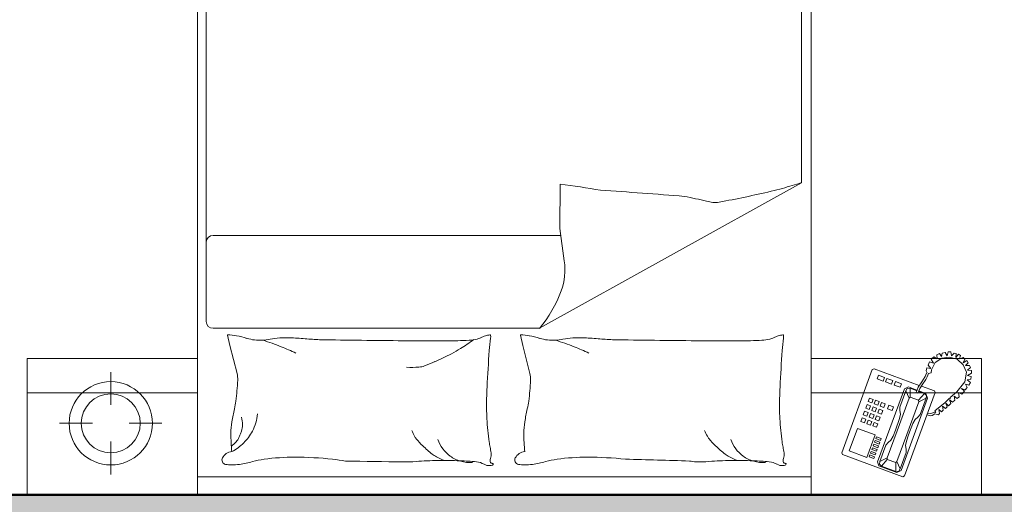
# Model space of a CAD drawing. Units: inches. Extents: x -7 to 1228, y -146 to 1091.
# Tile 66 of 88: x 656 to 745, y 573 to 617. Entities that reach past the tile are written whole.
import ezdxf

# ---------------------------------------------------------------- set-up
doc = ezdxf.new("R2010")
doc.units = ezdxf.units.IN
for name, color, linetype, lineweight in [('A-FURN', 8, 'Continuous', 18), ('A-WALL', 7, 'Continuous', 50), ('A-WALL-PATT', 251, 'Continuous', 13)]:
    doc.layers.add(name, color=color, linetype=linetype, lineweight=lineweight)
doc.styles.add('DIM_FONT', font='SIMPLEX.shx', dxfattribs={"width": 0.8})

# ---------------------------------------------------------------- blocks, each defined once
blk = doc.blocks.new('A$C4F634EDD')
for p, q in [((0, 2.6295), (0, 2.2295)), ((0.5, 2.6295), (0, 2.6295)), ((0.5, 2.6295), (2.3, 2.6295)), ((0.5, 0.5295), (0.5, 2.6295)), ((0.5, 2.2295), (0.5, 2.6295)), ((2.3, 2.6295), (2.3, 0.5295)), ((2.3, 2.6295), (2.8, 2.6295)), ((2.3, 2.2295), (2.3, 2.6295)), ((2.8, 2.6295), (2.8, 2.2295)), ((0.5, 2.5771), (2.3, 2.5771)), ((2.392, 2.5115), (2.5692, 2.5765)), ((2.5692, 2.5765), (2.574, 2.5743)), ((2.574, 2.5743), (2.6638, 2.3298)), ((0.2457, 2.5697), (0.2457, 2.4733)), ((2.4946, 2.5331), (2.4985, 2.5445)), ((2.4985, 2.5445), (2.5516, 2.564)), ((2.5062, 2.5454), (2.5004, 2.5392)), ((2.5062, 2.5454), (2.5487, 2.561)), ((2.5235, 2.5256), (2.5062, 2.5454)), ((2.5483, 2.5347), (2.5487, 2.561)), ((2.5487, 2.561), (2.5571, 2.56)), ((2.5615, 2.5536), (2.5514, 2.5318)), ((2.5516, 2.564), (2.5637, 2.5584)), ((2.5571, 2.56), (2.5615, 2.5536)), ((2.5615, 2.5536), (2.5791, 2.5058)), ((2.5637, 2.5584), (2.6418, 2.3458)), ((2.412, 2.5007), (2.4634, 2.5196)), ((2.4634, 2.5196), (2.4875, 2.454)), ((2.4842, 2.5232), (2.47, 2.518)), ((2.47, 2.518), (2.472, 2.5127)), ((2.472, 2.5127), (2.4862, 2.5179)), ((2.4862, 2.5179), (2.4842, 2.5232)), ((2.5734, 2.3187), (2.4946, 2.5331)), ((2.5004, 2.5392), (2.5013, 2.5315)), ((2.5013, 2.5315), (2.5188, 2.4836)), ((2.5013, 2.5315), (2.5231, 2.5214)), ((2.5231, 2.5214), (2.5235, 2.5256)), ((2.5523, 2.4417), (2.5231, 2.5214)), ((2.5483, 2.5347), (2.5235, 2.5256)), ((2.5514, 2.5318), (2.5483, 2.5347)), ((2.5807, 2.4521), (2.5514, 2.5318)), ((2.3898, 2.5066), (2.392, 2.5115)), ((2.4795, 2.2621), (2.3898, 2.5066)), ((2.4361, 2.4352), (2.412, 2.5007)), ((2.4881, 2.5126), (2.4739, 2.5074)), ((2.4739, 2.5074), (2.4759, 2.502)), ((2.4759, 2.502), (2.4901, 2.5073)), ((2.492, 2.5019), (2.4778, 2.4967)), ((2.4778, 2.4967), (2.4798, 2.4914)), ((2.4798, 2.4914), (2.494, 2.4966)), ((2.4959, 2.4913), (2.4817, 2.4861)), ((2.4817, 2.4861), (2.4837, 2.4808)), ((2.4837, 2.4808), (2.4979, 2.486)), ((2.4901, 2.5073), (2.4881, 2.5126)), ((2.494, 2.4966), (2.492, 2.5019)), ((2.4979, 2.486), (2.4959, 2.4913)), ((2.5788, 2.4956), (2.5767, 2.4848)), ((2.5767, 2.4848), (2.5795, 2.4717)), ((2.5791, 2.5058), (2.5788, 2.4956)), ((2.4998, 2.4807), (2.4856, 2.4755)), ((2.4856, 2.4755), (2.4876, 2.4702)), ((2.4876, 2.4702), (2.5018, 2.4754)), ((2.5037, 2.47), (2.4895, 2.4648)), ((2.4895, 2.4648), (2.4915, 2.4595)), ((2.4915, 2.4595), (2.5057, 2.4647)), ((2.5018, 2.4754), (2.4998, 2.4807)), ((2.5057, 2.4647), (2.5037, 2.47)), ((2.5188, 2.4836), (2.5256, 2.4761)), ((2.5256, 2.4761), (2.5342, 2.4692)), ((2.5342, 2.4692), (2.5405, 2.4574)), ((2.5405, 2.4574), (2.547, 2.4397)), ((2.5795, 2.4717), (2.586, 2.454)), ((2.4875, 2.454), (2.4361, 2.4352)), ((2.4811, 2.4276), (2.4917, 2.4315)), ((2.485, 2.4169), (2.4811, 2.4276)), ((2.4917, 2.4315), (2.4956, 2.4208)), ((2.5594, 2.4061), (2.547, 2.4397)), ((2.5523, 2.4417), (2.5875, 2.346)), ((2.5807, 2.4521), (2.6158, 2.3564)), ((2.5984, 2.4204), (2.586, 2.454)), ((0.0957, 2.4197), (0.192, 2.4197)), ((0.2994, 2.4197), (0.3957, 2.4197)), ((2.4457, 2.4146), (2.4563, 2.4185)), ((2.4496, 2.4039), (2.4457, 2.4146)), ((2.4602, 2.4078), (2.4496, 2.4039)), ((2.4528, 2.3951), (2.4635, 2.399)), ((2.4563, 2.4185), (2.4602, 2.4078)), ((2.4634, 2.4211), (2.474, 2.425)), ((2.4673, 2.4104), (2.4634, 2.4211)), ((2.4635, 2.399), (2.4674, 2.3883)), ((2.4779, 2.4143), (2.4673, 2.4104)), ((2.4706, 2.4016), (2.4812, 2.4055)), ((2.4745, 2.3909), (2.4706, 2.4016)), ((2.474, 2.425), (2.4779, 2.4143)), ((2.4812, 2.4055), (2.4851, 2.3949)), ((2.4956, 2.4208), (2.485, 2.4169)), ((2.4883, 2.4081), (2.4989, 2.412)), ((2.4922, 2.3975), (2.4883, 2.4081)), ((2.5028, 2.4014), (2.4922, 2.3975)), ((2.4989, 2.412), (2.5028, 2.4014)), ((2.5622, 2.393), (2.5594, 2.4061)), ((2.6047, 2.4086), (2.5984, 2.4204)), ((2.6133, 2.4017), (2.6047, 2.4086)), ((2.6201, 2.3941), (2.6133, 2.4017)), ((2.6499, 2.3979), (2.6397, 2.3953)), ((2.6551, 2.397), (2.6499, 2.3979)), ((2.4567, 2.3844), (2.4528, 2.3951)), ((2.4674, 2.3883), (2.4567, 2.3844)), ((2.46, 2.3756), (2.4706, 2.3795)), ((2.4639, 2.365), (2.46, 2.3756)), ((2.4745, 2.3689), (2.4639, 2.365)), ((2.4706, 2.3795), (2.4745, 2.3689)), ((2.4851, 2.3949), (2.4745, 2.3909)), ((2.4777, 2.3821), (2.4883, 2.386)), ((2.4816, 2.3715), (2.4777, 2.3821)), ((2.4922, 2.3754), (2.4816, 2.3715)), ((2.4883, 2.386), (2.4922, 2.3754)), ((2.4954, 2.3886), (2.5061, 2.3925)), ((2.4993, 2.378), (2.4954, 2.3886)), ((2.51, 2.3819), (2.4993, 2.378)), ((2.5026, 2.3691), (2.5132, 2.373)), ((2.5065, 2.3585), (2.5026, 2.3691)), ((2.5061, 2.3925), (2.51, 2.3819)), ((2.5132, 2.373), (2.5171, 2.3624)), ((2.5238, 2.3769), (2.538, 2.3821)), ((2.5277, 2.3663), (2.5238, 2.3769)), ((2.5419, 2.3715), (2.5277, 2.3663)), ((2.538, 2.3821), (2.5419, 2.3715)), ((2.5598, 2.372), (2.5601, 2.3822)), ((2.5774, 2.3242), (2.5598, 2.372)), ((2.5601, 2.3822), (2.5622, 2.393)), ((2.6376, 2.3463), (2.6201, 2.3941)), ((2.6417, 2.39), (2.6488, 2.391)), ((2.6488, 2.391), (2.6538, 2.3895)), ((2.6538, 2.3895), (2.6596, 2.388)), ((2.6627, 2.392), (2.6551, 2.397)), ((2.6596, 2.388), (2.6626, 2.3867)), ((2.6626, 2.3867), (2.6662, 2.388)), ((2.6692, 2.394), (2.6627, 2.392)), ((2.6662, 2.388), (2.6632, 2.3828)), ((2.6632, 2.3828), (2.6736, 2.3744)), ((2.6736, 2.3944), (2.6692, 2.394)), ((2.6765, 2.391), (2.6736, 2.3944)), ((2.6736, 2.3744), (2.6922, 2.3593)), ((2.6742, 2.3795), (2.6765, 2.391)), ((2.6824, 2.3858), (2.6742, 2.3795)), ((2.6873, 2.3815), (2.6824, 2.3858)), ((2.6853, 2.369), (2.6873, 2.3815)), ((2.6946, 2.376), (2.6853, 2.369)), ((2.6995, 2.3713), (2.6946, 2.376)), ((2.695, 2.3603), (2.6995, 2.3713)), ((0.2457, 2.366), (0.2457, 2.2697)), ((2.4672, 2.3561), (2.4778, 2.36)), ((2.4711, 2.3455), (2.4672, 2.3561)), ((2.4817, 2.3494), (2.4711, 2.3455)), ((2.4778, 2.36), (2.4817, 2.3494)), ((2.4849, 2.3626), (2.4955, 2.3665)), ((2.4888, 2.352), (2.4849, 2.3626)), ((2.4994, 2.3559), (2.4888, 2.352)), ((2.4955, 2.3665), (2.4994, 2.3559)), ((2.5171, 2.3624), (2.5065, 2.3585)), ((2.5774, 2.3242), (2.5875, 2.346)), ((2.5875, 2.346), (2.5905, 2.3431)), ((2.5905, 2.3431), (2.5901, 2.3168)), ((2.6154, 2.3522), (2.5905, 2.3431)), ((2.6158, 2.3564), (2.6154, 2.3522)), ((2.6154, 2.3522), (2.6327, 2.3324)), ((2.6376, 2.3463), (2.6158, 2.3564)), ((2.6418, 2.3458), (2.6369, 2.332)), ((2.6385, 2.3386), (2.6376, 2.3463)), ((2.6922, 2.3593), (2.7051, 2.3473)), ((2.7031, 2.3682), (2.695, 2.3603)), ((2.7096, 2.3616), (2.7031, 2.3682)), ((2.7051, 2.3473), (2.7079, 2.3475)), ((2.7062, 2.351), (2.7096, 2.3616)), ((2.7147, 2.3578), (2.7062, 2.351)), ((2.7079, 2.3475), (2.7079, 2.3443)), ((2.7079, 2.3443), (2.727, 2.3277)), ((2.7214, 2.3517), (2.7147, 2.3578)), ((2.7196, 2.34), (2.7214, 2.3517)), ((2.7286, 2.3466), (2.7196, 2.34)), ((2.7346, 2.3423), (2.7286, 2.3466)), ((2.732, 2.3295), (2.7346, 2.3423)), ((0, 2.3301), (0.5, 2.3301)), ((2.8, 2.3301), (2.3, 2.3301)), ((2.561, 2.3141), (2.5433, 2.3076)), ((2.5649, 2.3035), (2.561, 2.3141)), ((2.5855, 2.3131), (2.5734, 2.3187)), ((2.5818, 2.3178), (2.5774, 2.3242)), ((2.5901, 2.3168), (2.5818, 2.3178)), ((2.6104, 2.3222), (2.5855, 2.3131)), ((2.5901, 2.3168), (2.6097, 2.324)), ((2.613, 2.3312), (2.6077, 2.3293)), ((2.6077, 2.3293), (2.6135, 2.3141)), ((2.6192, 2.3174), (2.613, 2.3312)), ((2.6135, 2.3141), (2.6244, 2.2977)), ((2.6153, 2.3261), (2.6327, 2.3324)), ((2.6369, 2.332), (2.6161, 2.3243)), ((2.626, 2.3069), (2.6192, 2.3174)), ((2.6616, 2.3249), (2.6234, 2.3109)), ((2.6327, 2.3324), (2.6385, 2.3386)), ((2.6638, 2.3298), (2.6616, 2.3249)), ((2.727, 2.3277), (2.7512, 2.2983)), ((2.7423, 2.3345), (2.732, 2.3295)), ((2.7406, 2.3172), (2.7495, 2.325)), ((2.7519, 2.3218), (2.7406, 2.3172)), ((2.7495, 2.325), (2.7423, 2.3345)), ((2.7575, 2.3144), (2.7519, 2.3218)), ((2.7526, 2.3045), (2.7575, 2.3144)), ((2.6172, 2.3086), (2.4844, 2.2599)), ((2.5114, 2.2959), (2.4936, 2.2894)), ((2.4936, 2.2894), (2.4976, 2.2788)), ((2.4976, 2.2788), (2.5153, 2.2853)), ((2.5153, 2.2853), (2.5114, 2.2959)), ((2.5362, 2.305), (2.5185, 2.2985)), ((2.5185, 2.2985), (2.5224, 2.2879)), ((2.5224, 2.2879), (2.5401, 2.2944)), ((2.5401, 2.2944), (2.5362, 2.305)), ((2.5433, 2.3076), (2.5472, 2.297)), ((2.5472, 2.297), (2.5649, 2.3035)), ((2.6244, 2.2977), (2.6349, 2.2825)), ((2.6365, 2.2916), (2.626, 2.3069)), ((2.6349, 2.2825), (2.638, 2.273)), ((2.6407, 2.2834), (2.6365, 2.2916)), ((2.6438, 2.2739), (2.6407, 2.2834)), ((2.7512, 2.2983), (2.756, 2.2695)), ((2.7622, 2.308), (2.7526, 2.3045)), ((2.7574, 2.2924), (2.7673, 2.2997)), ((2.7687, 2.2905), (2.7574, 2.2924)), ((2.7587, 2.279), (2.7699, 2.2828)), ((2.7673, 2.2997), (2.7622, 2.308)), ((2.7699, 2.2828), (2.7687, 2.2905)), ((0.5953, 2.1912), (0.616, 2.2738)), ((1.4546, 2.1912), (1.4752, 2.2738)), ((2.4844, 2.2599), (2.4795, 2.2621)), ((2.6399, 2.2712), (2.6374, 2.2659)), ((2.6374, 2.2659), (2.6398, 2.257)), ((2.638, 2.273), (2.6399, 2.2712)), ((2.6398, 2.257), (2.6509, 2.259)), ((2.6509, 2.259), (2.6431, 2.2492)), ((2.6519, 2.2716), (2.6438, 2.2739)), ((2.6535, 2.2628), (2.6519, 2.2716)), ((2.6636, 2.2409), (2.6535, 2.2628)), ((2.756, 2.2695), (2.7459, 2.2483)), ((2.7708, 2.2725), (2.7587, 2.279)), ((2.759, 2.2637), (2.7706, 2.2643)), ((2.7676, 2.2559), (2.759, 2.2637)), ((2.7645, 2.2498), (2.7676, 2.2559)), ((2.7706, 2.2643), (2.7708, 2.2725)), ((0, 2.2295), (0.5, 2.2295)), ((2.8, 2.2295), (2.3, 2.2295)), ((2.6431, 2.2492), (2.6473, 2.2398)), ((2.6473, 2.2398), (2.6592, 2.2429)), ((2.6592, 2.2429), (2.6521, 2.2314)), ((2.6521, 2.2314), (2.6598, 2.2248)), ((2.6598, 2.2248), (2.6697, 2.2309)), ((2.6836, 2.2287), (2.6636, 2.2409)), ((2.6697, 2.2309), (2.6684, 2.219)), ((2.7063, 2.2256), (2.6836, 2.2287)), ((2.7284, 2.2317), (2.7063, 2.2256)), ((2.7255, 2.2152), (2.7242, 2.2265)), ((2.7242, 2.2265), (2.7324, 2.2165)), ((2.7459, 2.2483), (2.7284, 2.2317)), ((2.7386, 2.2208), (2.7354, 2.2306)), ((2.7354, 2.2306), (2.7462, 2.2264)), ((2.7509, 2.2314), (2.7459, 2.2418)), ((2.7459, 2.2418), (2.7568, 2.2352)), ((2.7462, 2.2264), (2.7509, 2.2314)), ((2.7529, 2.2505), (2.7645, 2.2498)), ((2.7607, 2.2424), (2.7529, 2.2505)), ((2.7568, 2.2352), (2.7607, 2.2424)), ((2.6684, 2.219), (2.6761, 2.2145)), ((2.6761, 2.2145), (2.6821, 2.2237)), ((2.6821, 2.2237), (2.6843, 2.2135)), ((2.6843, 2.2135), (2.6927, 2.2117)), ((2.6927, 2.2117), (2.6986, 2.222)), ((2.6986, 2.222), (2.7019, 2.2098)), ((2.7019, 2.2098), (2.7102, 2.2104)), ((2.7102, 2.2104), (2.7113, 2.2218)), ((2.7113, 2.2218), (2.7192, 2.2137)), ((2.7192, 2.2137), (2.7255, 2.2152)), ((2.7324, 2.2165), (2.7386, 2.2208)), ((0.5878, 2.1612), (0.5953, 2.1912)), ((1.4471, 2.1612), (1.4546, 2.1912)), ((1.5035, 2.141), (0.5458, 2.141)), ((1.5035, 2.141), (2.2716, 1.7136)), ((0.5258, 2.121), (0.5258, 0.5617)), ((1.576, 1.9433), (1.5624, 1.8479)), ((0.5458, 1.8684), (1.5653, 1.8684)), ((1.5624, 1.8479), (1.5641, 1.7178)), ((2.2716, 0.5617), (2.2716, 1.7136))]:
    blk.add_line(p, q)
for radius in [0.1222, 0.0865]:
    blk.add_circle((0.2457, 2.4197), radius)
for centre, radius, start, end in [((0.5999, 2.4516), 0.0904, 90, 101.2724), ((0.5999, 2.3808), 0.1611, 81.5628, 90), ((1.3554, 2.5152), 0.0289, 85.6975, 120.6513), ((1.3556, 2.519), 0.0251, 68.2117, 85.6975), ((1.3637, 2.5391), 0.00342, 19.564, 68.2117), ((1.4591, 2.4516), 0.0904, 90, 101.2724), ((1.4591, 2.3808), 0.1611, 81.5628, 90), ((2.2146, 2.5152), 0.0289, 85.6975, 120.6513), ((2.2149, 2.519), 0.0251, 68.2117, 85.6975), ((2.2229, 2.5391), 0.00342, 19.564, 68.2117), ((0.5848, 2.5274), 0.0131, 101.2724, 206.5805), ((0.6036, 2.5368), 0.0342, 206.5805, 265.5998), ((0.5788, 2.2388), 0.3048, 74.256, 81.5628), ((0.7272, 2.7653), 0.2422, 254.256, 262.4531), ((0.7851, 3.2019), 0.6827, 262.4531, 270), ((0.7851, 3.5682), 1.049, 270, 276.0867), ((0.8402, 3.0514), 0.5293, 276.0867, 280.1899), ((1.1602, -8.1346), 10.6675, 90.30153, 91.21582), ((1.1169, 2.2433), 0.2897, 85.1982, 92.5386), ((1.2142, 3.4021), 0.8732, 265.1982, 269.4243), ((1.2362, 2.45), 0.0768, 117.2396, 128.3886), ((1.3082, 2.3102), 0.234, 110.8603, 117.2396), ((1.2204, 4.0232), 1.4943, 269.4243, 271.9079), ((1.2995, 2.4357), 0.0992, 126.0864, 143.8234), ((1.2995, 2.4357), 0.0992, 105.9352, 126.0864), ((1.2429, 3.3501), 0.8208, 271.9079, 275.2592), ((1.2995, 2.4357), 0.0992, 85.7841, 105.9352), ((1.3132, 2.5864), 0.0539, 275.2592, 300.6513), ((1.3739, 2.5288), 0.0156, 158.0096, 201.421), ((1.3634, 2.533), 0.00428, 78.1069, 158.0096), ((1.3288, 2.5111), 0.0328, 351.8665, 21.421), ((1.3647, 2.5395), 0.00232, 258.1069, 19.564), ((1.444, 2.5274), 0.0131, 101.2724, 206.5805), ((1.4628, 2.5368), 0.0342, 206.5805, 265.5998), ((1.438, 2.2388), 0.3048, 74.256, 81.5628), ((1.5865, 2.7653), 0.2422, 254.256, 262.4531), ((1.6443, 3.2019), 0.6827, 262.4531, 270), ((1.6443, 3.5682), 1.049, 270, 276.0867), ((1.4785, 15.4878), 12.9656, 271.22425, 272.05324), ((1.97, 2.3805), 0.1524, 92.5386, 100.1899), ((1.9761, 2.2433), 0.2897, 85.1982, 92.5386), ((2.0734, 3.4021), 0.8732, 265.1982, 269.4243), ((2.0954, 2.45), 0.0768, 117.2396, 128.3886), ((2.1674, 2.3102), 0.234, 110.8603, 117.2396), ((2.0797, 4.0232), 1.4943, 269.4243, 271.9079), ((2.1588, 2.4357), 0.0992, 126.0864, 143.8234), ((2.1588, 2.4357), 0.0992, 105.9352, 126.0864), ((2.1021, 3.3501), 0.8208, 271.9079, 275.2592), ((2.1588, 2.4357), 0.0992, 85.7841, 105.9352), ((2.1724, 2.5864), 0.0539, 275.2592, 300.6513), ((2.2331, 2.5288), 0.0156, 158.0096, 201.421), ((2.2226, 2.533), 0.00428, 78.1069, 158.0096), ((2.1881, 2.5111), 0.0328, 351.8665, 21.421), ((2.224, 2.5395), 0.00232, 258.1069, 19.564), ((1.0898, 2.4496), 0.4918, 173.7676, 180), ((0.5462, 2.4142), 0.0899, 41.4429, 53.7359), ((0.5368, 2.3783), 0.1399, 45.0976, 62.7964), ((1.3165, 2.3233), 0.2252, 133.8115, 140.9651), ((1.4317, 2.2032), 0.3916, 128.3886, 133.8115), ((1.2995, 2.4357), 0.0992, 143.8234, 161.5603), ((1.5522, 2.448), 0.1983, 167.8905, 172.3191), ((1.1177, 2.5413), 0.246, 347.8905, 351.8665), ((1.949, 2.4496), 0.4918, 173.7676, 180), ((2.1757, 2.3233), 0.2252, 133.8115, 140.9651), ((2.291, 2.2032), 0.3916, 128.3886, 133.8115), ((2.1588, 2.4357), 0.0992, 143.8234, 161.5603), ((2.4114, 2.448), 0.1983, 167.8905, 172.3191), ((1.977, 2.5413), 0.246, 347.8905, 351.8665), ((0.5741, 2.4389), 0.0526, 25.3551, 41.4429), ((0.4851, 2.3967), 0.1511, 21.8149, 25.3551), ((0.5368, 2.3783), 0.1399, 27.3988, 45.0976), ((1.3127, 2.3625), 0.2002, 151.6832, 156.9972), ((1.1799, 2.4341), 0.0493, 140.9651, 151.6832), ((2.2605, 2.3525), 0.9131, 172.3191, 176.6313), ((2.1719, 2.3625), 0.2002, 151.6832, 156.9972), ((2.0391, 2.4341), 0.0493, 140.9651, 151.6832), ((3.1198, 2.3525), 0.9131, 172.3191, 176.6313), ((0.8019, 2.4496), 0.204, 180, 189.6844), ((0.4345, 2.3765), 0.2056, 18.7799, 21.8149), ((0.576, 2.4246), 0.0562, 0, 18.7799), ((0.5368, 2.3783), 0.1399, 16.515, 27.3988), ((1.6611, 2.4496), 0.204, 180, 189.6844), ((1.4703, 2.5637), 0.882, 189.6844, 192.1984), ((0.5406, 2.4246), 0.0915, 345.3149, 0), ((0.5368, 2.3783), 0.1399, 5.6311, 16.515), ((2.0266, 2.3663), 0.6787, 176.6313, 181.6331), ((2.3295, 2.5637), 0.882, 189.6844, 192.1984), ((2.8858, 2.3663), 0.6787, 176.6313, 181.6331), ((0.2982, 2.3103), 0.3171, 8.0051, 12.1984), ((1.1575, 2.3103), 0.3171, 8.0051, 12.1984), ((-0.0401, 2.2627), 0.6588, 2.6649, 8.0051), ((2.7128, 2.3859), 1.3652, 181.6331, 183.055), ((0.8191, 2.2627), 0.6588, 2.6649, 8.0051), ((3.5721, 2.3859), 1.3652, 181.6331, 183.055), ((14.9657, 3.0398), 13.6356, 183.05496, 183.50486), ((15.8249, 3.0398), 13.6356, 183.05496, 183.50486), ((0.5503, 2.2902), 0.0677, 345.9548, 2.6649), ((1.4096, 2.2902), 0.0677, 345.9548, 2.6649), ((1.1303, 1.9835), 0.2721, 85.9172, 93.5552), ((1.1455, 2.197), 0.058, 69.3257, 85.9172), ((0.9871, 1.7772), 0.5066, 65.6735, 69.3257), ((0.6058, 0.9338), 1.4323, 63.5015, 65.6735), ((0.473, 2.8815), 0.7387, 291.6577, 293.4844), ((0.473, 2.8815), 0.7387, 293.4844, 295.3111), ((1.1054, 1.9358), 0.3126, 57.865, 63.5015), ((0.8841, 1.5835), 0.7286, 54.1737, 57.865), ((1.6762, 2.2258), 0.3212, 183.5049, 189.9984), ((1.3322, 2.8815), 0.7387, 291.6577, 293.4844), ((1.3322, 2.8815), 0.7387, 293.4844, 295.3111), ((2.5355, 2.2258), 0.3212, 183.5049, 189.9984), ((0.5763, 2.3896), 0.2297, 279.4841, 287.3864), ((0.6807, 2.0561), 0.1197, 96.4341, 107.3864), ((0.6836, 2.0301), 0.1459, 78.4414, 96.4341), ((0.473, 2.8815), 0.7387, 287.1982, 289.428), ((0.759, 2.3985), 0.2301, 258.4414, 272.7491), ((0.473, 2.8815), 0.7387, 289.428, 291.6577), ((0.7026, 3.5718), 1.4048, 272.7491, 274.6176), ((0.9136, 0.9591), 1.2165, 92.6096, 94.6176), ((1.2501, -19.8405), 22.0183, 90.37908, 91.01965), ((1.2012, -3.5404), 5.7185, 89.7135, 90.9704), ((1.224, 1.0141), 1.164, 86.426, 89.7135), ((1.2875, 2.0302), 0.1459, 77.131, 86.426), ((1.3099, 2.1283), 0.0453, 62.7159, 77.131), ((1.3658, 2.2367), 0.0767, 242.7159, 253.7788), ((1.3409, 2.1667), 0.0193, 343.3022, 9.9984), ((1.4355, 2.3896), 0.2297, 279.4841, 287.3864), ((1.5399, 2.0561), 0.1197, 96.4341, 107.3864), ((1.5429, 2.0301), 0.1459, 78.4414, 96.4341), ((1.3322, 2.8815), 0.7387, 287.1982, 289.428), ((1.6182, 2.3985), 0.2301, 258.4414, 272.7491), ((1.3322, 2.8815), 0.7387, 289.428, 291.6577), ((1.5619, 3.5718), 1.4048, 272.7491, 274.6176), ((1.7729, 0.9591), 1.2165, 92.6096, 94.6176), ((2.1093, -19.8405), 22.0183, 90.37908, 91.01965), ((2.0605, -3.5404), 5.7185, 89.7135, 90.9704), ((2.0833, 1.0141), 1.164, 86.426, 89.7135), ((2.1467, 2.0302), 0.1459, 77.131, 86.426), ((2.1691, 2.1283), 0.0453, 62.7159, 77.131), ((2.2251, 2.2367), 0.0767, 242.7159, 253.7788), ((2.2001, 2.1667), 0.0193, 343.3022, 9.9984), ((0.5458, 2.121), 0.02, 90, 180), ((0.5887, 2.1609), 0.000917, 165.9551, 274.0829), ((0.5695, 2.4301), 0.2708, 274.0829, 279.4841), ((1.3688, 2.247), 0.0875, 253.7788, 262.8796), ((1.3581, 2.1615), 0.00132, 262.8796, 343.3022), ((1.448, 2.1609), 0.000917, 165.9551, 274.0829), ((1.4288, 2.4301), 0.2708, 274.0829, 279.4841), ((1.2147, 1.9017), 0.3751, 20.1488, 39.6445), ((2.2281, 2.247), 0.0875, 253.7788, 262.8796), ((2.2174, 2.1615), 0.00132, 262.8796, 343.3022), ((1.3977, 1.9688), 0.1801, 351.8644, 20.1488), ((0.5458, 1.8884), 0.02, 180, 270), ((1.4194, 4.2174), 2.5158, 281.6741, 283.1904), ((2.0378, 1.5789), 0.1942, 97.7304, 103.1904), ((2.0195, 1.7137), 0.0581, 79.2724, 97.7304), ((1.2737, -2.2227), 4.0646, 77.0745, 79.2724), ((1.0582, 5.4638), 3.7801, 277.692, 279.495), ((0.6102, 18.0525), 16.3521, 273.75703, 274.62393), ((2.0359, 1.0981), 0.6574, 74.0648, 77.0745), ((1.7125, -0.0344), 1.8351, 72.2636, 74.0648)]:
    blk.add_arc(centre, radius, start, end)
at = {"style": 'DIM_FONT', "width": 0.8, "flags": 9}
for tag, p in [('YSIZE', (0.5, 2.6295)), ('XSIZE', (0.5, 2.6295)), ('XSIZE', (2.2985, 2.6295)), ('YSIZE', (2.2985, 2.6295))]:
    blk.add_attdef(tag, p, '', height=0.0005, dxfattribs=at)

msp = doc.modelspace()

# ---------------------------------------------------------------- hatches: boundary and pattern name
at = {"layer": 'A-WALL-PATT'}
h = msp.add_hatch(color=256, dxfattribs=at)
h.dxf.hatch_style = 1
h.paths.add_polyline_path([(69, 568), (60, 568), (60, 493), (63.289, 493), (69, 493)])
h.paths.add_polyline_path([(69, 662.405), (60, 662.405), (60, 586), (69, 586)], flags=17)
h.paths.add_polyline_path([(69, 723), (184, 723), (184, 734), (179, 734), (179, 728), (69, 728), (69, 741.623), (60, 741.623), (60, 698.405), (69, 698.405)], flags=17)
h.paths.add_polyline_path([(69, 782), (231, 782), (231, 728), (231, 723), (231, 586), (236, 586), (236, 787), (69, 787), (69, 800.126), (60, 800.126), (60, 765.623), (69, 765.623)])
h.paths.add_polyline_path([(184, 842), (189, 842), (189, 848), (173, 848), (173, 842), (179, 842), (179, 787), (184, 787)])
h.paths.add_polyline_path([(118.22, 69), (69, 69), (69, 60), (118.22, 60)])
h.paths.add_polyline_path([(227, 69), (154.22, 69), (154.22, 60), (227, 60)])
h.paths.add_polyline_path([(236, 60), (232.711, 60), (227, 60), (227, 36), (236, 36)])
h.paths.add_polyline_path([(389, 60), (380, 60), (380, 36), (389, 36)])
h.paths.add_polyline_path([(384, 181), (380, 181), (380, 115), (380, 78), (384, 78)])
h.paths.add_polyline_path([(380, 115), (334.547, 115), (334.547, 109), (380, 109)])
h.paths.add_polyline_path([(274.547, 115), (236, 115), (236, 201), (232.711, 201), (231, 201), (231, 78), (236, 78), (236, 109), (274.547, 109)])
h.paths.add_polyline_path([(69, 123), (60, 123), (60, 78), (69, 78)])
h.paths.add_polyline_path([(69, 201), (60, 201), (60, 159), (69, 159)])
h.paths.add_polyline_path([(143, 219), (69, 219), (69, 213), (143, 213)], flags=17)
h.paths.add_polyline_path([(189, 219), (184, 219), (184, 274), (231, 274), (231, 219), (236, 219), (236, 279), (184, 279), (184, 297), (179, 297), (179, 279), (69, 279), (69, 290.912), (60, 290.912), (60, 262.179), (69, 262.179), (69, 274), (179, 274), (179, 219), (173, 219), (173, 213), (189, 213)])
h.paths.add_polyline_path([(69, 238.179), (60, 238.179), (60, 219), (69, 219)], flags=17)
h.paths.add_polyline_path([(69, 333), (60, 333), (60, 314.912), (69, 314.912), (69, 316.965)])
h.paths.add_polyline_path([(190, 338), (184, 338), (69, 338), (69, 333), (179, 333), (179, 327), (184, 327), (184, 333.021), (190, 333.046)])
h.paths.add_polyline_path([(69, 386.806), (60, 386.806), (60, 351), (69, 351)])
h.paths.add_polyline_path([(69, 475), (60, 475), (60, 422.806), (69, 422.806)])
h.paths.add_polyline_path([(236, 475), (231, 475), (231, 351.238), (236, 351.238)])
h.paths.add_polyline_path([(384, 475), (380, 475), (380, 362), (384, 362)])
h.paths.add_polyline_path([(547, 307), (439, 307), (439, 356), (445, 356), (445, 362), (433, 362), (433, 307), (380, 307), (380, 244), (380, 241), (384, 241), (384, 301), (433, 301), (433, 277), (439, 277), (439, 301), (547, 301)])
h.paths.add_polyline_path([(547, 241), (439, 241), (439, 247), (433, 247), (433, 235), (547, 235)])
h.paths.add_polyline_path([(450, 69), (440.286, 69), (424.889, 69), (389, 69), (389, 60), (450, 60)])
h.paths.add_polyline_path([(547, 69), (486, 69), (486, 60), (547, 60)])
h.paths.add_polyline_path([(556, 148.268), (547, 148.268), (547, 78), (556, 78)])
h.paths.add_polyline_path([(556, 223), (547, 223), (547, 195), (547, 184.268), (556, 184.268)])
h.paths.add_polyline_path([(556, 311.192), (547, 311.192), (547, 273.075), (556, 273.075)])
h.paths.add_polyline_path([(556, 344), (552.711, 344), (547, 344), (547, 335.192), (556, 335.192)])
h.paths.add_polyline_path([(556, 249.075), (547, 249.075), (547, 241), (556, 241)])
h.paths.add_polyline_path([(547, 362), (475, 362), (475, 356), (547, 356)], flags=0)
h.paths.add_polyline_path([(556, 399.621), (547, 399.621), (547, 362), (556, 362)])
h.paths.add_polyline_path([(556, 475), (547, 475), (547, 435.621), (556, 435.621)])
h.paths.add_polyline_path([(547, 493), (389, 493), (389, 487), (547, 487)])
h.paths.add_polyline_path([(380, 493), (278, 493), (278, 487), (380, 487)])
h.paths.add_polyline_path([(227, 493), (69, 493), (69, 487), (227, 487)])
h.paths.add_polyline_path([(643, 122.445), (634, 122.445), (634, 78), (643, 78)])
h.paths.add_polyline_path([(702.5, 69), (692.786, 69), (677.389, 69), (643, 69), (643, 60), (702.5, 60)])
h.paths.add_polyline_path([(798, 69), (738.5, 69), (738.5, 60), (798, 60)])
h.paths.add_polyline_path([(807, 60), (803.711, 60), (798, 60), (798, 36), (807, 36)])
h.paths.add_polyline_path([(807, 109), (846.751, 109), (846.751, 115), (807, 115), (807, 159), (802, 159), (802, 78), (807, 78)])
h.paths.add_polyline_path([(807, 201), (802, 201), (802, 195), (807, 195)])
h.paths.add_polyline_path([(643, 201), (634, 201), (634, 158.445), (643, 158.445)])
h.paths.add_polyline_path([(756, 225), (751, 225), (751, 219), (643, 219), (643, 213), (756, 213)])
h.paths.add_polyline_path([(643, 240.848), (634, 240.848), (634, 219), (643, 219)])
h.paths.add_polyline_path([(643, 274), (643, 288.629), (634, 288.629), (634, 264.848), (643, 264.848)])
h.paths.add_polyline_path([(802, 279), (756, 279), (756, 297), (751, 297), (751, 279), (643, 279), (643, 274), (751, 274), (751, 255), (756, 255), (756, 274), (802, 274)])
h.paths.add_polyline_path([(807, 333), (803.711, 333), (802, 333), (802, 279), (802, 274), (802, 219), (807, 219)])
h.paths.add_polyline_path([(956, 182), (951, 182), (951, 115), (906.751, 115), (906.751, 109), (951, 109), (951, 78), (956, 78)])
h.paths.add_polyline_path([(960, 60), (951, 60), (951, 36), (960, 36)])
h.paths.add_polyline_path([(1021, 69), (1005.781, 69), (960, 69), (960, 60), (1021, 60)])
h.paths.add_polyline_path([(956, 224), (951, 224), (951, 218), (956, 218)])
h.paths.add_polyline_path([(956, 302), (1004, 302), (1004, 278), (1010, 278), (1010, 302), (1118, 302), (1118, 290.809), (1127, 290.809), (1127, 326.968), (1118, 326.968), (1118, 320.966), (1118, 307), (1010, 307), (1010, 356), (1016, 356), (1016, 362), (1004, 362), (1004, 307), (951, 307), (951, 244), (951, 242), (954.289, 242), (956, 242)])
h.paths.add_polyline_path([(643, 333), (634, 333), (634, 312.629), (643, 312.629), (643, 316.965)])
h.paths.add_polyline_path([(756, 338), (643, 338), (643, 333), (751, 333), (751, 327), (756, 327)])
h.paths.add_polyline_path([(643, 388), (634, 388), (634, 351), (643, 351)])
h.paths.add_polyline_path([(807, 357), (802, 357), (802, 351), (807, 351)])
h.paths.add_polyline_path([(807, 475), (802, 475), (802, 393), (807, 393)])
h.paths.add_polyline_path([(643, 475), (634, 475), (634, 424), (643, 424)])
h.paths.add_polyline_path([(798, 493), (643, 493), (643, 487), (798, 487)])
h.paths.add_polyline_path([(634, 493), (556, 493), (556, 487), (634, 487)])
h.paths.add_polyline_path([(813, 493), (807, 493), (807, 487), (813, 487)])
h.paths.add_polyline_path([(951, 493), (849, 493), (849, 487), (951, 487)])
h.paths.add_polyline_path([(956, 484), (951, 484), (951, 374), (956, 374)])
h.paths.add_polyline_path([(1109, 493), (969, 493), (969, 487), (1109, 487)])
h.paths.add_polyline_path([(1127, 484), (1118, 484), (1118, 450.641), (1127, 450.641)])
h.paths.add_polyline_path([(1127, 414.641), (1118, 414.641), (1118, 365), (1127, 365)])
h.paths.add_polyline_path([(1109, 362), (1046, 362), (1046, 356), (1109, 356)], flags=17)
h.paths.add_polyline_path([(1127, 356), (1123.454, 356), (1118, 356), (1118, 350.968), (1127, 350.968)], flags=0)
h.paths.add_polyline_path([(1127, 266.809), (1118, 266.809), (1118, 262.361), (1118, 242), (1127, 242)], flags=17)
h.paths.add_polyline_path([(1118, 242), (1010, 242), (1010, 248), (1004, 248), (1004, 237), (1118, 237)])
h.paths.add_polyline_path([(1127, 224), (1118, 224), (1118, 170), (1127, 170)])
h.paths.add_polyline_path([(1127, 134), (1118, 134), (1118, 78), (1127, 78)])
h.paths.add_polyline_path([(1118, 69), (1057, 69), (1057, 60), (1118, 60)])
h.paths.add_polyline_path([(227, 571.546), (227, 574), (69, 574), (69, 568), (227, 568)])
h.paths.add_polyline_path([(380, 571.546), (380, 574), (278, 574), (278, 568), (380, 568)])
h.paths.add_polyline_path([(242, 574), (236, 574), (236, 568), (242, 568)])
h.paths.add_polyline_path([(547, 571.546), (547, 574), (389, 574), (389, 568), (547, 568)])
h.paths.add_polyline_path([(384, 733), (380, 733), (380, 586), (384, 586)])
h.paths.add_polyline_path([(556, 646), (634, 646), (634, 655), (547, 655), (547, 586), (556, 586)])
h.paths.add_polyline_path([(634, 574), (556, 574), (556, 568), (634, 568)])
h.paths.add_polyline_path([(643, 655), (634, 655), (634, 586), (643, 586)])
h.paths.add_polyline_path([(798, 574), (643, 574), (643, 568), (798, 568)])
h.paths.add_polyline_path([(643, 663.854), (634, 663.854), (634, 655), (643, 655)])
h.paths.add_polyline_path([(556, 676.967), (547, 676.967), (547, 655), (556, 655)])
h.paths.add_polyline_path([(556, 733), (547, 733), (547, 712.967), (556, 712.967)])
h.paths.add_polyline_path([(643, 710), (634, 710), (634, 699.854), (643, 699.854)])
h.paths.add_polyline_path([(807, 668), (802, 668), (802, 586), (807, 586)])
h.paths.add_polyline_path([(951, 574), (849, 574), (849, 568), (951, 568)])
h.paths.add_polyline_path([(956, 691), (951, 691), (951, 577), (956, 577)])
h.paths.add_polyline_path([(1109, 574), (969, 574), (969, 568), (1109, 568)])
h.paths.add_polyline_path([(1127, 643.403), (1118, 643.403), (1118, 577), (1127, 577)])
h.paths.add_polyline_path([(1127, 568), (1123.454, 568), (1118, 568), (1118, 493), (1127, 493)])
h.paths.add_polyline_path([(1127, 733), (1118, 733), (1118, 679.403), (1127, 679.403)])
h.paths.add_polyline_path([(1127, 777.348), (1118, 777.348), (1118, 770.035), (1118, 751), (1127, 751)], flags=17)
h.paths.add_polyline_path([(1118, 751), (1010, 751), (1010, 757), (1004, 757), (1004, 745), (1118, 745)])
h.paths.add_polyline_path([(956, 811), (1004, 811), (1004, 787), (1010, 787), (1010, 811), (1017.874, 811), (1017.874, 811.627, -0.414214), (1018.247, 812), (1031.978, 812, -0.414214), (1032.351, 811.627), (1032.351, 811), (1118, 811), (1118, 801.348), (1127, 801.348), (1127, 834.685), (1118, 834.685), (1118, 830.238), (1118, 817), (1010, 817), (1010, 866), (1016, 866), (1016, 872), (1004, 872), (1004, 817), (956, 817), (956, 866), (951, 866), (951, 751), (954.289, 751), (956, 751)])
h.paths.add_polyline_path([(1118, 872), (1046, 872), (1046, 866), (1118, 866)], flags=17)
h.paths.add_polyline_path([(1127, 924.711), (1118, 924.711), (1118, 884), (1127, 884)])
h.paths.add_polyline_path([(1127, 866), (1123.711, 866), (1118, 866), (1118, 858.685), (1127, 858.685)], flags=17)
h.paths.add_polyline_path([(956, 983), (951, 983), (951, 952), (807, 952), (807, 983), (802, 983), (802, 902), (807, 902), (807, 946), (951, 946), (951, 884), (956, 884)])
h.paths.add_polyline_path([(807, 842), (802, 842), (802, 787), (756, 787), (756, 806), (751, 806), (751, 787), (643, 787), (643, 782), (751, 782), (751, 764), (756, 764), (756, 782), (802, 782), (802, 728), (807, 728)])
h.paths.add_polyline_path([(756, 848), (643, 848), (643, 842), (751, 842), (751, 836), (756, 836)])
h.paths.add_polyline_path([(756, 734), (751, 734), (751, 728), (643, 728), (643, 723), (756, 723)])
h.paths.add_polyline_path([(643, 749.791), (634, 749.791), (634, 728), (637.289, 728), (643, 728)])
h.paths.add_polyline_path([(643, 805.405), (634, 805.405), (634, 773.791), (643, 773.791)])
h.paths.add_polyline_path([(643, 896.663), (634, 896.663), (634, 860), (637.289, 860), (643, 860)])
h.paths.add_polyline_path([(643, 842), (634, 842), (634, 829.405), (643, 829.405)])
h.paths.add_polyline_path([(643, 983), (634, 983), (634, 932.663), (643, 932.663)])
h.paths.add_polyline_path([(1127, 983), (1118, 983), (1118, 960.711), (1127, 960.711)])
h.paths.add_polyline_path([(1118, 1001), (1077.525, 1001), (1077.525, 992), (1118, 992)])
h.paths.add_polyline_path([(1041.525, 1001), (960, 1001), (960, 992), (1041.525, 992)])
h.paths.add_polyline_path([(960, 1025), (951, 1025), (951, 1001), (954.289, 1001), (960, 1001)])
h.paths.add_polyline_path([(807, 1025), (798, 1025), (798, 1001), (807, 1001)])
h.paths.add_polyline_path([(798, 1001), (738.5, 1001), (738.5, 992), (798, 992)])
h.paths.add_polyline_path([(702.5, 1001), (643, 1001), (643, 992), (702.5, 992)])
h.paths.add_polyline_path([(547, 1001), (499.113, 1001), (499.113, 992), (547, 992)])
h.paths.add_polyline_path([(463.113, 1001), (389, 1001), (389, 992), (463.113, 992)])
h.paths.add_polyline_path([(389, 1025), (380, 1025), (380, 1022), (380, 1001), (383.289, 1001), (389, 1001)])
h.paths.add_polyline_path([(236, 1025), (227, 1025), (227, 1001), (236, 1001)])
h.paths.add_polyline_path([(236, 983), (231, 983), (231, 860), (236, 860)])
h.paths.add_polyline_path([(274.547, 952), (236, 952), (236, 946), (274.547, 946)])
h.paths.add_polyline_path([(380, 952), (334.547, 952), (334.547, 946), (380, 946)])
h.paths.add_polyline_path([(384, 983), (380, 983), (380, 884), (383.289, 884), (384, 884)])
h.paths.add_polyline_path([(227, 1001), (155.012, 1001), (155.012, 992), (162.875, 992), (227, 992)])
h.paths.add_polyline_path([(119.012, 1001), (69, 1001), (69, 992), (119.012, 992)])
h.paths.add_polyline_path([(69, 983), (60, 983), (60, 922.987), (69, 922.987)])
h.paths.add_polyline_path([(69, 886.987), (60, 886.987), (60, 860), (63.289, 860), (69, 860)])
h.paths.add_polyline_path([(143, 848), (69, 848), (69, 842), (143, 842)])

# ---------------------------------------------------------------- linework, layer by layer
at = {"layer": 'A-WALL'}
msp.add_line((813, 574), (556, 574), dxfattribs=at)

# ---------------------------------------------------------------- block references
at = {"layer": 'A-FURN', "xscale": -30.79356024027943, "yscale": 30.79356024027943, "zscale": 30.79356024027943, "rotation": 180}
msp.add_blockref('A$C4F634EDD', (656.965, 654.972), dxfattribs=at)

doc.saveas('drawing.dxf')
